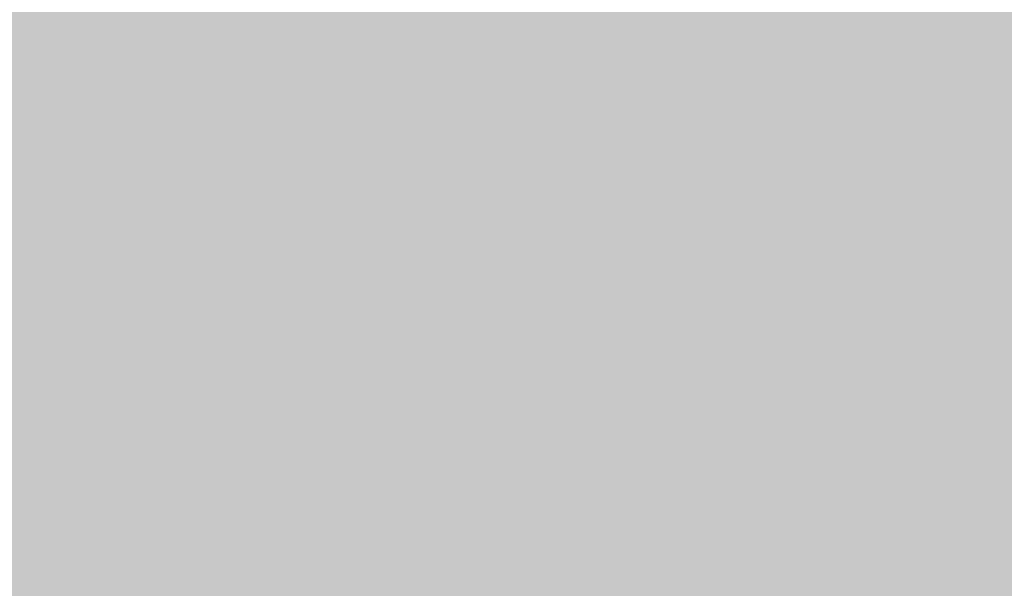
# Model space of a CAD drawing. Units: inches. Extents: x 2696 to 3240, y 1564 to 2310.
# Tile 55 of 76: x 2907.148 to 2916.848, y 2179.88 to 2185.477. Entities that reach past the tile are written whole.
import ezdxf

# ---------------------------------------------------------------- set-up
doc = ezdxf.new("R2010")
doc.units = ezdxf.units.IN
doc.layers.add('A-ANNO-DIMS', color=3, linetype='Continuous', lineweight=18)
doc.layers.add('A-WALL-PATT', color=9, linetype='Continuous', lineweight=13)
doc.styles.add('TIMES NEW', font='times.ttf')
doc.dimstyles.new('Siddhuu', dxfattribs={"dimtxt": 6, "dimasz": 2.5, "dimexe": 1.25, "dimexo": 0.625, "dimtad": 1, "dimdec": 1, "dimlunit": 4, "dimtxsty": 'TIMES NEW', "dimcen": 2.5, "dimclrd": 256, "dimclre": 1, "dimclrt": 7, "dimadec": 0, "dimazin": 0, "dimtfac": 1, "dimtdec": 1, "dimtmove": 0, "dimatfit": 3, "dimfxl": 1, "dimtolj": 1, "dimlwd": -1, "dimarcsym": 0})

# ---------------------------------------------------------------- blocks, each defined once
blk = doc.blocks.new('*D59')
at = {"layer": 'A-ANNO-DIMS', "color": 1, "lineweight": -2, "transparency": 16777216}
for p, q in [((2884.7088, 1740.8261), (2884.7088, 2298.4511)), ((2956.7088, 1740.8261), (2956.7088, 2298.4511))]:
    blk.add_line(p, q, dxfattribs=at)
at = {"layer": 'A-ANNO-DIMS', "transparency": 16777216}
blk.add_line((2887.2088, 2297.2011), (2954.2088, 2297.2011), dxfattribs=at)
for points in [[(2887.2088, 2297.6178), (2887.2088, 2296.7844), (2884.7088, 2297.2011)], [(2954.2088, 2297.6178), (2954.2088, 2296.7844), (2956.7088, 2297.2011)]]:
    blk.add_solid(points, dxfattribs=at)
at = {"layer": 'Defpoints', "color": 0, "transparency": 16777216}
for p in [(2956.7088, 2297.2011), (2884.7088, 1740.2011), (2956.7088, 1740.2011)]:
    blk.add_point(p, dxfattribs=at)
at = {"layer": 'A-ANNO-DIMS', "color": 7, "transparency": 16777216, "insert": (2920.7088, 2300.878), "char_height": 6, "attachment_point": 5, "style": 'TIMES NEW'}
blk.add_mtext('\\A1;6\'-0"', dxfattribs=at)
blk = doc.blocks.new('*D64')
at = {"layer": 'A-ANNO-DIMS', "color": 1, "lineweight": -2, "transparency": 16777216}
for p, q in [((3073.0838, 2206.7011), (2709.3614, 2206.7011)), ((3068.5838, 1989.2011), (2709.3614, 1989.2011))]:
    blk.add_line(p, q, dxfattribs=at)
at = {"layer": 'A-ANNO-DIMS', "transparency": 16777216}
blk.add_line((2710.6114, 1991.7011), (2710.6114, 2204.2011), dxfattribs=at)
for points in [[(2710.1947, 2204.2011), (2711.0281, 2204.2011), (2710.6114, 2206.7011)], [(2710.1947, 1991.7011), (2711.0281, 1991.7011), (2710.6114, 1989.2011)]]:
    blk.add_solid(points, dxfattribs=at)
at = {"layer": 'Defpoints', "color": 0, "transparency": 16777216}
for p in [(2710.6114, 2206.7011), (3073.7088, 2206.7011), (3069.2088, 1989.2011)]:
    blk.add_point(p, dxfattribs=at)
at = {"layer": 'A-ANNO-DIMS', "color": 7, "transparency": 16777216, "insert": (2706.8501, 2097.9511), "char_height": 6, "attachment_point": 5, "rotation": 90, "style": 'TIMES NEW'}
blk.add_mtext('\\A1;18\'-1 1/2"', dxfattribs=at)

msp = doc.modelspace()

# ---------------------------------------------------------------- hatches: boundary and pattern name
at = {"layer": 'A-WALL-PATT', "transparency": 33554556}
h = msp.add_hatch(color=256, dxfattribs=at)
h.dxf.hatch_style = 1
h.paths.add_polyline_path([(2879.1114, 2253.2011), (2905.9101, 2253.2011), (2905.9101, 2262.2011), (2841.889, 2262.2011), (2841.889, 2253.2011), (2870.1114, 2253.2011), (2870.1114, 2176.6011), (2965.7088, 2176.6011), (2965.7088, 2206.7011), (2973.5828, 2206.7011), (2973.5828, 2215.7011), (2965.7088, 2215.7011), (2965.7088, 2262.2011), (2929.9101, 2262.2011), (2929.9101, 2253.2011), (2956.7088, 2253.2011), (2956.7088, 2185.6011), (2879.1114, 2185.6011)])
h.paths.add_polyline_path([(2782.8338, 2262.2011), (2745.6114, 2262.2011), (2745.6114, 2228.7287), (2754.6114, 2228.7287), (2754.6114, 2253.2011), (2782.8338, 2253.2011)])
h.paths.add_polyline_path([(2754.6114, 2136.2011), (2965.7088, 2136.2011), (2965.7088, 2145.2011), (2879.1114, 2145.2011), (2879.1114, 2147.0735), (2877.3397, 2147.0735), (2870.1114, 2147.0735), (2870.1114, 2145.2011), (2754.6114, 2145.2011), (2754.6114, 2169.6735), (2745.6114, 2169.6735), (2745.6114, 2000.2011), (2754.6114, 2000.2011), (2754.6114, 2019.2011), (2849.0828, 2019.2011), (2849.0828, 2023.7011), (2841.2088, 2023.7011), (2841.2088, 2051.8271), (2836.7088, 2051.8271), (2836.7088, 2023.7011), (2754.6114, 2023.7011), (2754.6114, 2091.2011), (2836.7088, 2091.2011), (2836.7088, 2087.8271), (2841.2088, 2087.8271), (2841.2088, 2095.7011), (2754.6114, 2095.7011)])
h.paths.add_polyline_path([(2965.7088, 2136.2011), (2956.7088, 2136.2011), (2956.7088, 2023.7011), (2885.0828, 2023.7011), (2885.0828, 2019.2011), (2956.7088, 2019.2011), (2956.7088, 1950.5751), (2965.7088, 1950.5751), (2965.7088, 1980.2011), (2973.5828, 1980.2011), (2973.5828, 1989.2011), (2965.7088, 1989.2011)])
h.paths.add_polyline_path([(2754.6114, 1906.7011), (2880.2088, 1906.7011), (2884.7088, 1906.7011), (2956.7088, 1906.7011), (2956.7088, 1792.7011), (2944.7088, 1792.7011), (2944.7088, 1783.7011), (2956.7088, 1783.7011), (2956.7088, 1740.2011), (2884.7088, 1740.2011), (2884.7088, 1783.7011), (2896.7088, 1783.7011), (2896.7088, 1792.7011), (2884.7088, 1792.7011), (2884.7088, 1846.7011), (2880.2088, 1846.7011), (2880.2088, 1740.2011), (2754.6114, 1740.2011), (2754.6114, 1777.2011), (2745.6114, 1777.2011), (2745.6114, 1692.7011), (2754.6114, 1692.7011), (2754.6114, 1731.2011), (2956.7088, 1731.2011), (2956.7088, 1723.3271), (2965.7088, 1723.3271), (2965.7088, 1884.2011), (2973.5828, 1884.2011), (2973.5828, 1893.2011), (2965.7088, 1893.2011), (2965.7088, 1914.5751), (2956.7088, 1914.5751), (2956.7088, 1911.2011), (2754.6114, 1911.2011), (2754.6114, 1930.2011), (2745.6114, 1930.2011), (2745.6114, 1817.2011), (2754.6114, 1817.2011), (2754.6114, 1854.2011), (2826.6114, 1854.2011), (2826.6114, 1868.8271), (2822.1114, 1868.8271), (2822.1114, 1858.7011), (2754.6114, 1858.7011)])
h.paths.add_polyline_path([(2965.7088, 1656.2011), (3008.2374, 1656.2011), (3008.2374, 1665.2011), (2965.7088, 1665.2011), (2965.7088, 1693.3271), (2956.7088, 1693.3271), (2956.7088, 1686.2011), (2934.5828, 1686.2011), (2934.5828, 1681.7011), (2956.7088, 1681.7011), (2956.7088, 1614.2011), (2896.7088, 1614.2011), (2896.7088, 1681.7011), (2904.5828, 1681.7011), (2904.5828, 1686.2011), (2892.2088, 1686.2011), (2892.2088, 1614.2011), (2858.4101, 1614.2011), (2858.4101, 1605.2011), (2965.7088, 1605.2011)])
h.paths.add_polyline_path([(2788.4101, 1614.2011), (2754.6114, 1614.2011), (2754.6114, 1652.7011), (2745.6114, 1652.7011), (2745.6114, 1605.2011), (2788.4101, 1605.2011)])
h.paths.add_polyline_path([(3199.6114, 1633.0476), (3190.6114, 1633.0476), (3190.6114, 1614.2011), (3082.6114, 1614.2011), (3082.6114, 1665.2011), (3070.2374, 1665.2011), (3070.2374, 1656.2011), (3078.1114, 1656.2011), (3078.1114, 1605.2011), (3199.6114, 1605.2011)])
h.paths.add_polyline_path([(3199.6114, 1702.0476), (3190.6114, 1702.0476), (3190.6114, 1699.7011), (3106.6114, 1699.7011), (3106.6114, 1747.7011), (3190.6114, 1747.7011), (3190.6114, 1752.2011), (3082.6114, 1752.2011), (3082.6114, 1760.0751), (3078.1114, 1760.0751), (3078.1114, 1747.7011), (3102.1114, 1747.7011), (3102.1114, 1699.7011), (3078.1114, 1699.7011), (3078.1114, 1695.2011), (3190.6114, 1695.2011), (3190.6114, 1676.3546), (3199.6114, 1676.3546)])
h.paths.add_polyline_path([(3199.6114, 1783.2011), (3190.6114, 1783.2011), (3190.6114, 1745.3546), (3199.6114, 1745.3546)])
h.paths.add_polyline_path([(3082.6114, 1884.2011), (3190.6114, 1884.2011), (3190.6114, 1853.2011), (3199.6114, 1853.2011), (3199.6114, 1901.7011), (3190.6114, 1901.7011), (3190.6114, 1893.2011), (3005.5828, 1893.2011), (3005.5828, 1891.2811), (3005.5828, 1884.2011), (3078.1114, 1884.2011), (3078.1114, 1792.0751), (3082.6114, 1792.0751)])
h.paths.add_polyline_path([(3199.6114, 1994.7011), (3190.6114, 1994.7011), (3190.6114, 1989.2011), (3073.7088, 1989.2011), (3073.7088, 2034.2011), (3069.2088, 2034.2011), (3069.2088, 1989.2011), (3005.5828, 1989.2011), (3005.5828, 1980.2011), (3190.6114, 1980.2011), (3190.6114, 1971.7011), (3199.6114, 1971.7011)])
h.paths.add_polyline_path([(3199.6114, 2155.2011), (3190.6114, 2155.2011), (3190.6114, 2064.7011), (3199.6114, 2064.7011)])
h.paths.add_polyline_path([(3190.6114, 2074.7011), (3106.6114, 2074.7011), (3106.6114, 2122.7011), (3190.6114, 2122.7011), (3190.6114, 2127.2011), (3082.7088, 2127.2011), (3082.7088, 2135.0751), (3073.7088, 2135.0751), (3073.7088, 2122.7011), (3102.1114, 2122.7011), (3102.1114, 2074.7011), (3069.2088, 2074.7011), (3069.2088, 2070.2011), (3190.6114, 2070.2011)])
h.paths.add_polyline_path([(3082.7088, 2253.2011), (3190.6114, 2253.2011), (3190.6114, 2225.2011), (3199.6114, 2225.2011), (3199.6114, 2262.2011), (3073.7088, 2262.2011), (3073.7088, 2215.7011), (3035.5828, 2215.7011), (3035.5828, 2206.7011), (3073.7088, 2206.7011), (3073.7088, 2171.0751), (3082.7088, 2171.0751)])

# ---------------------------------------------------------------- dimensions: what is measured, and where the dimension line sits
at = {"layer": 'A-ANNO-DIMS'}
dim = msp.add_linear_dim(base=(2956.7088, 2297.2011), p1=(2884.7088, 1740.2011), p2=(2956.7088, 1740.2011), dimstyle='Siddhuu', override={"dimdec": 1, "dimlfac": 1, "dimrnd": 0, "dimzin": 1, "dimdsep": 46, "dimlunit": 4, "dimfrac": 2}, dxfattribs=at)
dim.commit()
dim.dimension.update_dxf_attribs({"geometry": '*D59', "text_midpoint": (2920.7088, 2300.878)})
dim = msp.add_linear_dim(base=(2710.6114, 2206.7011), p1=(3069.2088, 1989.2011), p2=(3073.7088, 2206.7011), angle=90, dimstyle='Siddhuu', override={"dimdec": 1, "dimlfac": 1, "dimrnd": 0, "dimzin": 1, "dimdsep": 46, "dimlunit": 4, "dimfrac": 2}, dxfattribs=at)
dim.commit()
dim.dimension.update_dxf_attribs({"geometry": '*D64', "text_midpoint": (2706.8501, 2097.9511)})

doc.saveas('drawing.dxf')
